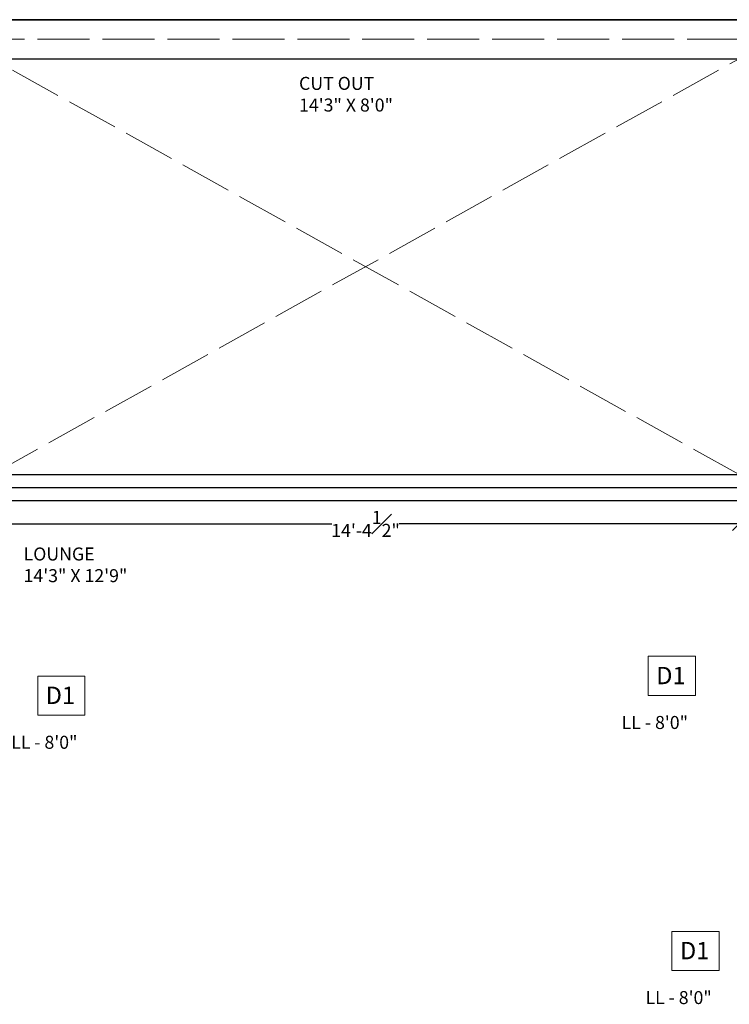
# Model space of a CAD drawing. Units: inches. Extents: x 1365 to 2091, y 1589 to 2091.
# Tile 5 of 8: x 1654 to 1818, y 1836 to 2063. Entities that reach past the tile are written whole.
import ezdxf

# ---------------------------------------------------------------- set-up
doc = ezdxf.new("R2010")
doc.units = ezdxf.units.IN
doc.linetypes.add('ACAD_ISO02W100', pattern=[15, 12, -3])
for name, color, linetype, lineweight in [('A-ANNO-DIMS', 2, 'Continuous', 18), ('A-ANNO-SYMB', 12, 'Continuous', 18), ('A-AREA-IDEN', 7, 'Continuous', 18), ('A-FLOR-HRAL', 7, 'Continuous', 25), ('A-FLOR-OPEN', 7, 'Continuous', 25), ('A-FLOR-OPEN-HIDN', 1, 'ACAD_ISO02W100', 18), ('A-WALL', 7, 'Continuous', 35)]:
    doc.layers.add(name, color=color, linetype=linetype, lineweight=lineweight)
doc.styles.get("Standard").update_dxf_attribs({"font": 'arial.ttf'})
doc.dimstyles.new('ISO-25', dxfattribs={"dimtxt": 3, "dimasz": 3, "dimexe": 1.25, "dimexo": 0.625, "dimtad": 0, "dimlunit": 4, "dimtxsty": 'Standard', "dimblk": 'OBLIQUE', "dimcen": 2.5, "dimclrd": 254, "dimclre": 254, "dimclrt": 1, "dimadec": 0, "dimazin": 0, "dimtfac": 1, "dimtmove": 0, "dimatfit": 3, "dimfxl": 1, "dimfxlon": 1, "dimfrac": 1, "dimarcsym": 0})

# ---------------------------------------------------------------- blocks, each defined once
blk = doc.blocks.new('_Oblique')
at = {"color": 0, "linetype": 'ByBlock', "lineweight": -2}
blk.add_line((-0.5, -0.5), (0.5, 0.5), dxfattribs=at)
blk = doc.blocks.new('*D93')
at = {"layer": 'A-ANNO-DIMS', "color": 0, "lineweight": -2, "transparency": 16777216}
for p, q in [((1647.25, 1947.47), (1647.25, 1945.22)), ((1647.25, 1946.47), (1725.72, 1946.47)), ((1819.75, 1946.47), (1741.29, 1946.47)), ((1819.75, 1947.47), (1819.75, 1945.22))]:
    blk.add_line(p, q, dxfattribs=at)
at = {"layer": 'Defpoints', "color": 0, "transparency": 16777216}
for p in [(1647.25, 1951.86), (1819.75, 1951.86), (1819.75, 1946.47)]:
    blk.add_point(p, dxfattribs=at)
at = {"layer": 'A-ANNO-DIMS', "color": 0, "lineweight": -2, "transparency": 16777216, "xscale": 3, "yscale": 3, "zscale": 3, "rotation": 180}
blk.add_blockref('_Oblique', (1647.25, 1946.47), dxfattribs=at)
at = {"layer": 'A-ANNO-DIMS', "color": 0, "lineweight": -2, "transparency": 16777216, "xscale": 3, "yscale": 3, "zscale": 3}
blk.add_blockref('_Oblique', (1819.75, 1946.47), dxfattribs=at)
at = {"layer": 'A-ANNO-DIMS', "color": 0, "transparency": 16777216, "insert": (1733.5, 1946.47), "char_height": 3, "attachment_point": 5}
blk.add_mtext('14\'-4{\\H1x;\\S1#2;}"', dxfattribs=at)
blk = doc.blocks.new('OPENING-TAG-D1')
blk.add_lwpolyline([(6.13, 13.79), (17.02, 13.79), (17.02, 4.75), (6.13, 4.75)], close=True)
at = {"attachment_point": 1}
for s, width, insert, char_height in [('{D1}', 14.5136, (7.98, 11.34), 4), ('{LL - 8\'0"}', 24.3857, (0, 0), 3)]:
    blk.add_mtext_dynamic_manual_height_columns(s, width=width, gutter_width=12.5, heights=[0], dxfattribs=dict(at, insert=insert, char_height=char_height))

msp = doc.modelspace()

# ---------------------------------------------------------------- linework, layer by layer
at = {"layer": 'A-FLOR-HRAL'}
for p, q in [((1647.254, 1957.858), (1819.754, 1957.858)), ((1647.254, 1954.858), (1819.754, 1954.858)), ((1647.254, 1951.858), (1819.754, 1951.858))]:
    msp.add_line(p, q, dxfattribs=at)
at = {"layer": 'A-FLOR-OPEN'}
msp.add_line((1647.254, 2053.858), (1819.754, 2053.858), dxfattribs=at)
at = {"layer": 'A-FLOR-OPEN-HIDN'}
for p, q in [((1819.754, 2058.358), (1647.254, 2058.358)), ((1819.754, 1957.858), (1647.254, 2053.858)), ((1647.254, 1957.858), (1819.754, 2053.858))]:
    msp.add_line(p, q, dxfattribs=at)
at = {"layer": 'A-WALL'}
msp.add_line((1393.754, 2062.858), (2053.754, 2062.858), dxfattribs=at)

# ---------------------------------------------------------------- block references
at = {"layer": 'A-ANNO-SYMB'}
for p in [(1792.651, 1902.122), (1651.651, 1897.551), (1798.133, 1838.615)]:
    msp.add_blockref('OPENING-TAG-D1', p, dxfattribs=at)

# ---------------------------------------------------------------- texts
at = {"layer": 'A-AREA-IDEN', "char_height": 3, "attachment_point": 1}
for s, insert in [('{CUT OUT\\P14\'3" X 8\'0"}', (1718.14, 2049.655)), ('{LOUNGE\\P14\'3" X 12\'9"}', (1654.529, 1941.015))]:
    msp.add_mtext_dynamic_manual_height_columns(s, width=33.58604, gutter_width=12.5, heights=[0], dxfattribs=dict(at, insert=insert))

# ---------------------------------------------------------------- dimensions: what is measured, and where the dimension line sits
at = {"layer": 'A-ANNO-DIMS'}
dim = msp.add_linear_dim(base=(1819.754, 1946.468), p1=(1647.254, 1951.858), p2=(1819.754, 1951.858), dimstyle='ISO-25', override={"dimclrd": 0, "dimclre": 0, "dimclrt": 0}, dxfattribs=at)
dim.commit()
dim.dimension.update_dxf_attribs({"geometry": '*D93', "text_midpoint": (1733.504, 1946.468)})

doc.saveas('drawing.dxf')
